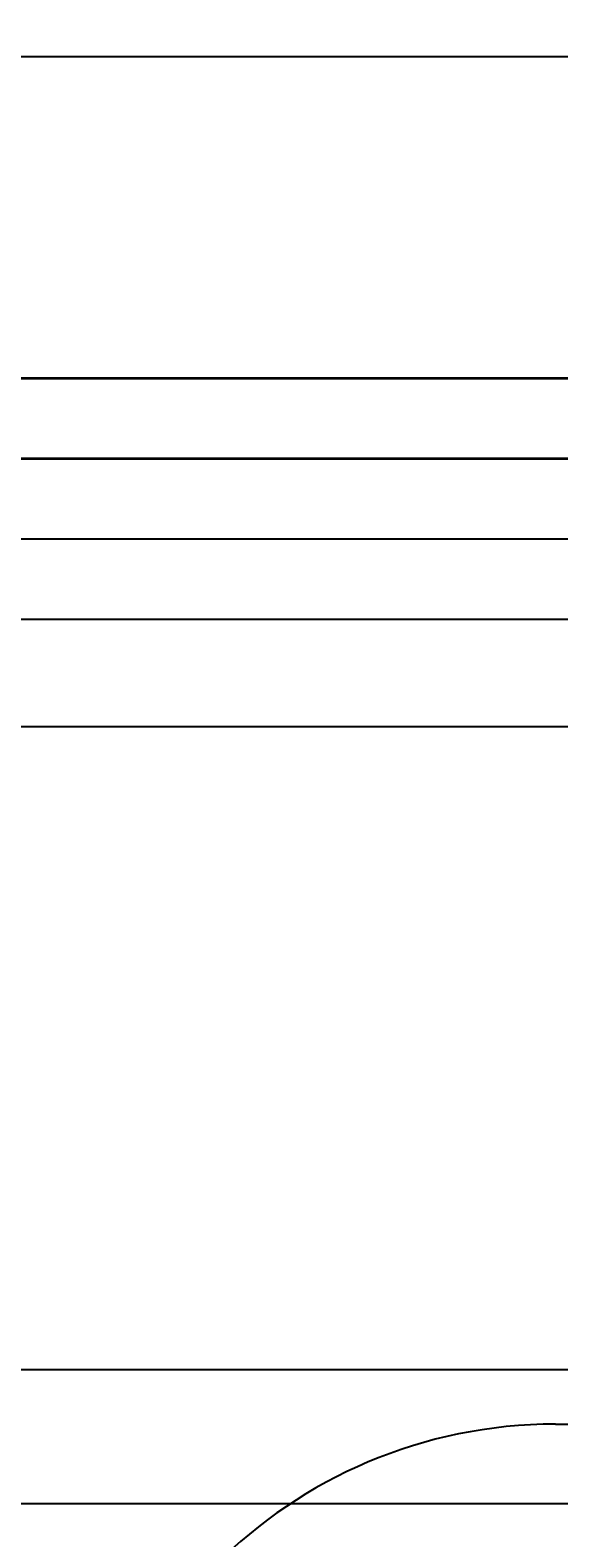
# Model space of a CAD drawing. Units: feet. Extents: x 105 to 1094, y -88 to 588.
# Tile 6 of 59: x 248 to 288, y 138 to 250. Entities that reach past the tile are written whole.
import ezdxf

# ---------------------------------------------------------------- set-up
doc = ezdxf.new("R2010")
doc.units = ezdxf.units.FT
doc.header["$MEASUREMENT"] = 0
for name, color, linetype, lineweight in [('A-ANNO-DIMS', 2, 'Continuous', 18), ('A-DOOR', 3, 'Continuous', 25), ('A-WALL', 7, 'Continuous', 35)]:
    doc.layers.add(name, color=color, linetype=linetype, lineweight=lineweight)
doc.styles.get("Standard").update_dxf_attribs({"font": 'arial.ttf'})
doc.dimstyles.get("Standard").update_dxf_attribs({"dimtxt": 0.18, "dimasz": 0.18, "dimexe": 0.18, "dimexo": 0.0625, "dimgap": 0.09, "dimtad": 0, "dimtih": 1, "dimtoh": 1, "dimdec": 4, "dimzin": 0, "dimdsep": 46, "dimtxsty": 'Standard', "dimcen": 0.09, "dimadec": 0, "dimazin": 0, "dimtfac": 1, "dimtdec": 4, "dimtofl": 0, "dimtmove": 0, "dimatfit": 3, "dimfxl": 1, "dimtolj": 1, "dimtzin": 0, "dimarcsym": 0})

# ---------------------------------------------------------------- blocks, each defined once
blk = doc.blocks.new('*U2')
for p, q in [((0, 0), (0, -6)), ((40, 0), (40, -6))]:
    blk.add_line(p, q)
blk.add_lwpolyline([(0, 0), (0, 40), (1.75, 40), (1.75, 0)], close=True)
blk.add_arc((0, 0), 40, 0, 90)
blk = doc.blocks.new('*D20')
at = {"layer": 'A-ANNO-DIMS', "color": 0, "lineweight": -2, "transparency": 16777216}
for p, q in [((150.69, 276.02), (150.69, -88.15)), ((1048.69, 276.02), (1048.69, -88.15)), ((150.87, -87.97), (599.4, -87.97)), ((1048.51, -87.97), (599.98, -87.97))]:
    blk.add_line(p, q, dxfattribs=at)
at = {"layer": 'A-ANNO-DIMS', "color": 0, "transparency": 16777216}
for points in [[(150.87, -87.94), (150.87, -88), (150.69, -87.97)], [(1048.51, -87.94), (1048.51, -88), (1048.69, -87.97)]]:
    blk.add_solid(points, dxfattribs=at)
at = {"layer": 'Defpoints', "color": 0, "transparency": 16777216}
for p in [(150.69, 276.08), (1048.69, 276.08), (1048.69, -87.97)]:
    blk.add_point(p, dxfattribs=at)
at = {"layer": 'A-ANNO-DIMS', "color": 0, "transparency": 16777216, "insert": (599.69, -87.97), "char_height": 0.18, "attachment_point": 5}
blk.add_mtext('\\A1;898', dxfattribs=at)
blk = doc.blocks.new('*D21')
at = {"layer": 'A-ANNO-DIMS', "color": 0, "lineweight": -2, "transparency": 16777216}
for p, q in [((849.63, 543.08), (105.46, 543.08)), ((105.64, 542.9), (105.64, 250.26)), ((105.64, -42.74), (105.64, 249.9)), ((849.63, -42.92), (105.46, -42.92))]:
    blk.add_line(p, q, dxfattribs=at)
at = {"layer": 'A-ANNO-DIMS', "color": 0, "transparency": 16777216}
for points in [[(105.61, 542.9), (105.67, 542.9), (105.64, 543.08)], [(105.61, -42.74), (105.67, -42.74), (105.64, -42.92)]]:
    blk.add_solid(points, dxfattribs=at)
at = {"layer": 'Defpoints', "color": 0, "transparency": 16777216}
for p in [(105.64, 543.08), (849.69, 543.08), (849.69, -42.92)]:
    blk.add_point(p, dxfattribs=at)
at = {"layer": 'A-ANNO-DIMS', "color": 0, "transparency": 16777216, "insert": (105.64, 250.08), "char_height": 0.18, "attachment_point": 5}
blk.add_mtext('\\A1;586', dxfattribs=at)
blk = doc.blocks.new('*D36')
at = {"layer": 'A-ANNO-DIMS', "color": 0, "lineweight": -2, "transparency": 16777216}
for p, q in [((547.24, 248.08), (105.46, 248.08)), ((105.64, 247.9), (105.64, 230.26)), ((105.64, 212.26), (105.64, 229.9)), ((546.63, 212.08), (105.46, 212.08))]:
    blk.add_line(p, q, dxfattribs=at)
at = {"layer": 'A-ANNO-DIMS', "color": 0, "transparency": 16777216}
for points in [[(105.61, 247.9), (105.67, 247.9), (105.64, 248.08)], [(105.61, 212.26), (105.67, 212.26), (105.64, 212.08)]]:
    blk.add_solid(points, dxfattribs=at)
at = {"layer": 'Defpoints', "color": 0, "transparency": 16777216}
for p in [(105.64, 248.08), (547.3, 248.08), (546.69, 212.08)]:
    blk.add_point(p, dxfattribs=at)
at = {"layer": 'A-ANNO-DIMS', "color": 0, "transparency": 16777216, "insert": (105.64, 230.08), "char_height": 0.18, "attachment_point": 5}
blk.add_mtext('\\A1;36', dxfattribs=at)
blk = doc.blocks.new('*D38')
at = {"layer": 'A-ANNO-DIMS', "color": 0, "lineweight": -2, "transparency": 16777216}
for p, q in [((150.69, 224.14), (150.69, 588.31)), ((150.87, 588.13), (222.41, 588.13)), ((294.51, 588.13), (222.97, 588.13)), ((294.69, 224.14), (294.69, 588.31))]:
    blk.add_line(p, q, dxfattribs=at)
at = {"layer": 'A-ANNO-DIMS', "color": 0, "transparency": 16777216}
for points in [[(150.87, 588.16), (150.87, 588.1), (150.69, 588.13)], [(294.51, 588.16), (294.51, 588.1), (294.69, 588.13)]]:
    blk.add_solid(points, dxfattribs=at)
at = {"layer": 'Defpoints', "color": 0, "transparency": 16777216}
for p in [(294.69, 588.13), (150.69, 224.08), (294.69, 224.08)]:
    blk.add_point(p, dxfattribs=at)
at = {"layer": 'A-ANNO-DIMS', "color": 0, "transparency": 16777216, "insert": (222.69, 588.13), "char_height": 0.18, "attachment_point": 5}
blk.add_mtext('\\A1;144', dxfattribs=at)
blk = doc.blocks.new('*D46')
at = {"layer": 'A-ANNO-DIMS', "color": 0, "lineweight": -2, "transparency": 16777216}
for p, q in [((580.63, 206.08), (105.46, 206.08)), ((105.64, 205.9), (105.64, 173.26)), ((105.64, 140.26), (105.64, 172.9)), ((580.63, 140.08), (105.46, 140.08))]:
    blk.add_line(p, q, dxfattribs=at)
at = {"layer": 'A-ANNO-DIMS', "color": 0, "transparency": 16777216}
for points in [[(105.61, 205.9), (105.67, 205.9), (105.64, 206.08)], [(105.61, 140.26), (105.67, 140.26), (105.64, 140.08)]]:
    blk.add_solid(points, dxfattribs=at)
at = {"layer": 'Defpoints', "color": 0, "transparency": 16777216}
for p in [(580.69, 206.08), (105.64, 140.08), (580.69, 140.08)]:
    blk.add_point(p, dxfattribs=at)
at = {"layer": 'A-ANNO-DIMS', "color": 0, "transparency": 16777216, "insert": (105.64, 173.08), "char_height": 0.18, "attachment_point": 5}
blk.add_mtext('\\A1;66', dxfattribs=at)
blk = doc.blocks.new('*D55')
at = {"layer": 'A-ANNO-DIMS', "color": 0, "lineweight": -2, "transparency": 16777216}
for p, q in [((292.63, 198.08), (105.46, 198.08)), ((105.64, 197.9), (105.64, 174.26)), ((105.64, 150.26), (105.64, 173.9)), ((293.13, 150.08), (105.46, 150.08))]:
    blk.add_line(p, q, dxfattribs=at)
at = {"layer": 'A-ANNO-DIMS', "color": 0, "transparency": 16777216}
for points in [[(105.61, 197.9), (105.67, 197.9), (105.64, 198.08)], [(105.61, 150.26), (105.67, 150.26), (105.64, 150.08)]]:
    blk.add_solid(points, dxfattribs=at)
at = {"layer": 'Defpoints', "color": 0, "transparency": 16777216}
for p in [(105.64, 198.08), (292.69, 198.08), (293.2, 150.08)]:
    blk.add_point(p, dxfattribs=at)
at = {"layer": 'A-ANNO-DIMS', "color": 0, "transparency": 16777216, "insert": (105.64, 174.08), "char_height": 0.18, "attachment_point": 5}
blk.add_mtext('\\A1;48', dxfattribs=at)

msp = doc.modelspace()

# ---------------------------------------------------------------- linework, layer by layer
at = {"layer": 'A-WALL'}
for p, q in [((294.6883, 224.0812), (150.6883, 224.0812)), ((288.6883, 218.0812), (156.6883, 218.0812))]:
    msp.add_line(p, q, dxfattribs=at)

# ---------------------------------------------------------------- block references
at = {"layer": 'A-DOOR', "xscale": 0.8984622266767051, "yscale": 0.8984622266767051, "zscale": 0.8984622266767051, "rotation": 90.00000000000003}
msp.add_blockref('*U2', (287.2975, 110.0812), dxfattribs=at)

# ---------------------------------------------------------------- dimensions: what is measured, and where the dimension line sits
at = {"layer": 'A-ANNO-DIMS'}
for base, p1, p2, picture, middle in [((294.6883, 588.1312), (150.6883, 224.0812), (294.6883, 224.0812), '*D38', (222.6883, 588.1312)), ((1048.6883, -87.9688), (150.6883, 276.0812), (1048.6883, 276.0812), '*D20', (599.6883, -87.9688))]:
    dim = msp.add_linear_dim(base=base, p1=p1, p2=p2, dimstyle='Standard', override={"dimdec": 0, "dimlfac": 1, "dimrnd": 0, "dimzin": 0, "dimdsep": 46, "dimlunit": 2}, dxfattribs=at)
    dim.commit()
    dim.dimension.update_dxf_attribs({"geometry": picture, "text_midpoint": middle})
for base, p1, p2, picture, middle in [((105.6383, 543.0812), (849.6883, -42.9188), (849.6883, 543.0812), '*D21', (105.6383, 250.0812)), ((105.6383, 248.0812), (546.6883, 212.0812), (547.2975, 248.0812), '*D36', (105.6383, 230.0812)), ((105.6383, 140.0812), (580.6883, 206.0812), (580.6883, 140.0812), '*D46', (105.6383, 173.0812)), ((105.6383, 198.0812), (293.1967, 150.0812), (292.6883, 198.0812), '*D55', (105.6383, 174.0812))]:
    dim = msp.add_linear_dim(base=base, p1=p1, p2=p2, angle=90, dimstyle='Standard', override={"dimdec": 0, "dimlfac": 1, "dimrnd": 0, "dimzin": 0, "dimdsep": 46, "dimlunit": 2}, dxfattribs=at)
    dim.commit()
    dim.dimension.update_dxf_attribs({"geometry": picture, "text_midpoint": middle})

doc.saveas('drawing.dxf')
